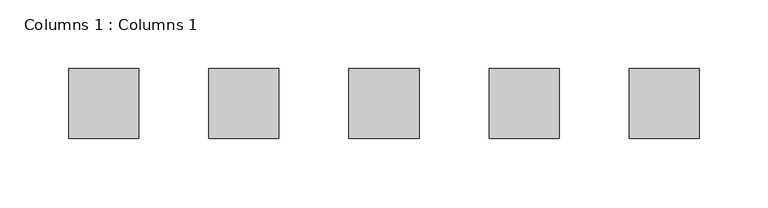
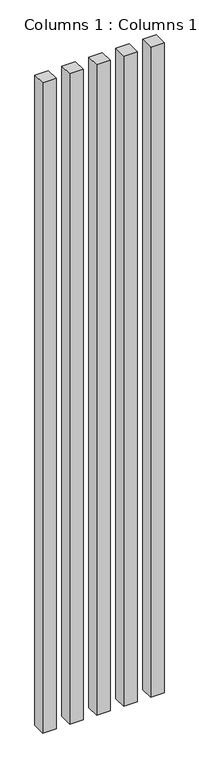
"""IFC4 building model written with IfcOpenShell, lengths in millimetres: column geometry, Columns 1 : Columns 1."""

from ifc_helpers import new_model, si_unit, frame, origin, place, context, project, spatial, polyline, outline, extrude, source, transform, mapped, element, save


def columns_1_columns_1_0c675057(model_context):
    return source(origin(), model_context, "Body", "SweptSolid", [
        extrude(outline(polyline([(-5264.4301496, -1885.997359), (-5264.4301496, -1835.197359), (-5213.6301496, -1835.197359), (-5213.6301496, -1885.997359), (-5264.4301496, -1885.997359)])), frame((0.0, 0.0, 3657.6), z_axis=(0.0, 0.0, 1.0), x_axis=(1.0, 0.0, 0.0)), (0.0, 0.0, 1.0), 2590.8),
        extrude(outline(polyline([(-5162.8301496, -1885.997359), (-5162.8301496, -1835.197359), (-5112.0301496, -1835.197359), (-5112.0301496, -1885.997359), (-5162.8301496, -1885.997359)])), frame((0.0, 0.0, 3657.6), z_axis=(0.0, 0.0, 1.0), x_axis=(1.0, 0.0, 0.0)), (0.0, 0.0, 1.0), 2590.8),
        extrude(outline(polyline([(-5061.2301496, -1885.997359), (-5061.2301496, -1835.197359), (-5010.4301496, -1835.197359), (-5010.4301496, -1885.997359), (-5061.2301496, -1885.997359)])), frame((0.0, 0.0, 3657.6), z_axis=(0.0, 0.0, 1.0), x_axis=(1.0, 0.0, 0.0)), (0.0, 0.0, 1.0), 2590.8),
        extrude(outline(polyline([(-4959.6301496, -1885.997359), (-4959.6301496, -1835.197359), (-4908.8301496, -1835.197359), (-4908.8301496, -1885.997359), (-4959.6301496, -1885.997359)])), frame((0.0, 0.0, 3657.6), z_axis=(0.0, 0.0, 1.0), x_axis=(1.0, 0.0, 0.0)), (0.0, 0.0, 1.0), 2590.8),
        extrude(outline(polyline([(-4858.0301496, -1885.997359), (-4858.0301496, -1835.197359), (-4807.2301496, -1835.197359), (-4807.2301496, -1885.997359), (-4858.0301496, -1885.997359)])), frame((0.0, 0.0, 3657.6), z_axis=(0.0, 0.0, 1.0), x_axis=(1.0, 0.0, 0.0)), (0.0, 0.0, 1.0), 2590.8),
    ])


if __name__ == "__main__":
    model = new_model("IFC4")
    model_context = context("Model", 3, world=origin())
    ifc_project = project(units=[si_unit("LENGTHUNIT", "METRE", prefix="MILLI")], contexts=[model_context])
    site = spatial("IfcSite", under=ifc_project)
    building = spatial("IfcBuilding", under=site)
    placement = place(None, origin())
    columns_1_columns_1_shape = columns_1_columns_1_0c675057(model_context)
    element("IfcColumn", 1, ObjectType="Columns 1 : Columns 1", at=placement, inside=building, context=model_context, shape_type="MappedRepresentation", body=[
        mapped(columns_1_columns_1_shape, transform((0.0, 0.0, 0.0), x_axis=(1.0, 0.0, 0.0), y_axis=(0.0, 1.0, 0.0), z_axis=(0.0, 0.0, 1.0))),
    ])
    save(model, "model.ifc")

# Revit data of these elements
# Element 1 (IfcColumn, "Columns 1 : Columns 1")
#   Materials on its faces: "Damp-proofing"
# Materials
#   "Damp-proofing": class "Generic", colour RGB 127 127 127, transparency 0, Description = "Damp-proofing", Cost = 0
